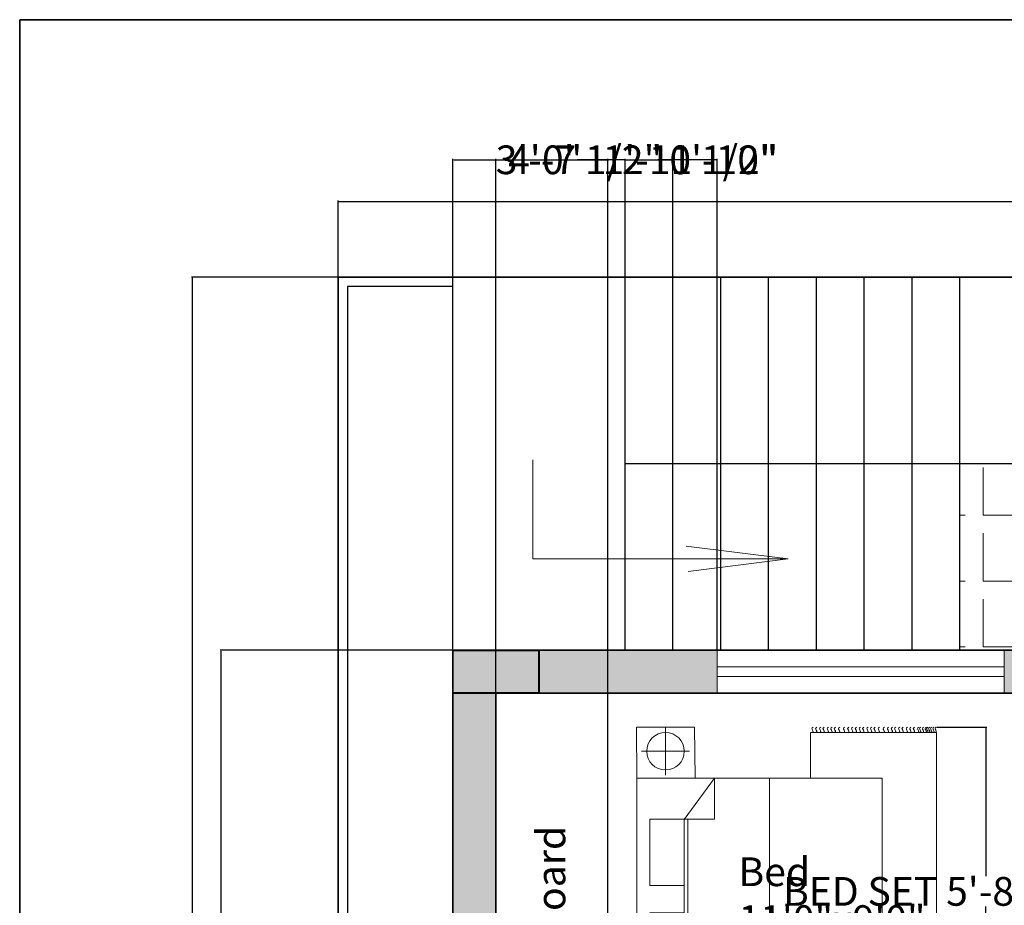
# Model space of a CAD drawing. Units: inches. Extents: x 56944 to 57417, y 173916 to 174454.
# Tile 7 of 8: x 56944 to 57149, y 174268 to 174454. Entities that reach past the tile are written whole.
import ezdxf

# ---------------------------------------------------------------- set-up
doc = ezdxf.new("R2010")
doc.units = ezdxf.units.IN
doc.header["$MEASUREMENT"] = 0
for name, color, linetype, lineweight in [('A-ANNO-DIMS', 2, 'Continuous', 18), ('A-ANNO-SYMB', 7, 'Continuous', 18), ('A-ANNO-TEXT', 7, 'Continuous', 18), ('A-ANNO-TTLB', 7, 'Continuous', 35), ('A-AREA-IDEN', 7, 'Continuous', 20), ('A-COLS', 7, 'Continuous', 40), ('A-COLS-PATT', 250, 'Continuous', 9), ('A-FLOR-CASE', 8, 'Continuous', 25), ('A-FLOR-STRS', 7, 'Continuous', 25), ('A-FURN', 8, 'Continuous', 18), ('A-GLAZ', 4, 'Continuous', 18), ('A-SITE-PATT', 8, 'Continuous', 9), ('A-SITE-WALL', 7, 'Continuous', 25), ('A-WALL', 7, 'Continuous', 35), ('A-WALL-PATT', 241, 'Continuous', 9), ('C-PROP', 7, 'Continuous', 35)]:
    doc.layers.add(name, color=color, linetype=linetype, lineweight=lineweight)
doc.styles.get("Standard").update_dxf_attribs({"font": 'arial.ttf'})
doc.dimstyles.get("Standard").update_dxf_attribs({"dimtxt": 6, "dimasz": 0.18, "dimexe": 0.18, "dimexo": 0.0625, "dimgap": 0.09, "dimtad": 0, "dimtih": 1, "dimtoh": 1, "dimdec": 1, "dimzin": 0, "dimdsep": 46, "dimlunit": 3, "dimtxsty": 'Standard', "dimcen": 0.09, "dimadec": 0, "dimazin": 0, "dimtfac": 1, "dimtdec": 1, "dimtofl": 0, "dimtmove": 0, "dimatfit": 3, "dimfxl": 1, "dimtolj": 1, "dimtzin": 0, "dimarcsym": 0})

# ---------------------------------------------------------------- blocks, each defined once
blk = doc.blocks.new('*D3')
at = {"layer": 'A-ANNO-DIMS', "color": 0, "lineweight": -2, "transparency": 16777216}
for p, q in [((57010.13, 174399.89), (57010.13, 174415.81)), ((57368.63, 174399.89), (57368.63, 174415.81)), ((57010.31, 174415.63), (57184.2, 174415.63)), ((57368.45, 174415.63), (57194.56, 174415.63))]:
    blk.add_line(p, q, dxfattribs=at)
at = {"layer": 'A-ANNO-DIMS', "color": 0, "transparency": 16777216}
for points in [[(57010.31, 174415.66), (57010.31, 174415.6), (57010.13, 174415.63)], [(57368.45, 174415.66), (57368.45, 174415.6), (57368.63, 174415.63)]]:
    blk.add_solid(points, dxfattribs=at)
at = {"layer": 'Defpoints', "color": 0, "transparency": 16777216}
for p in [(57368.63, 174415.63), (57010.13, 174399.82), (57368.63, 174399.82)]:
    blk.add_point(p, dxfattribs=at)
at = {"layer": 'A-ANNO-DIMS', "color": 0, "transparency": 16777216, "insert": (57189.38, 174415.63), "char_height": 6, "attachment_point": 5}
blk.add_mtext("\\A1;30'", dxfattribs=at)
blk = doc.blocks.new('*D4')
at = {"layer": 'A-ANNO-DIMS', "color": 0, "lineweight": -2, "transparency": 16777216}
for p, q in [((57010.07, 174399.82), (56979.48, 174399.82)), ((56979.66, 174399.64), (56979.66, 174183.23)), ((56979.66, 173960.5), (56979.66, 174176.92)), ((57010.07, 173960.32), (56979.48, 173960.32))]:
    blk.add_line(p, q, dxfattribs=at)
at = {"layer": 'A-ANNO-DIMS', "color": 0, "transparency": 16777216}
for points in [[(56979.63, 174399.64), (56979.69, 174399.64), (56979.66, 174399.82)], [(56979.63, 173960.5), (56979.69, 173960.5), (56979.66, 173960.32)]]:
    blk.add_solid(points, dxfattribs=at)
at = {"layer": 'Defpoints', "color": 0, "transparency": 16777216}
for p in [(57010.13, 174399.82), (56979.66, 173960.32), (57010.13, 173960.32)]:
    blk.add_point(p, dxfattribs=at)
at = {"layer": 'A-ANNO-DIMS', "color": 0, "transparency": 16777216, "insert": (56979.66, 174180.07), "char_height": 6, "width": 27.5975, "attachment_point": 5}
blk.add_mtext("\\A1;40'", dxfattribs=at)
blk = doc.blocks.new('BED-DOUBLE-WITH-NIGHTSTANDS')
for p, q in [((6.09, 68.68), (6.09, 58.62)), ((36.42, 67.59), (62.78, 67.59)), ((36.42, 58.05), (36.42, 67.59)), ((62.78, 67.59), (62.78, 4.35)), ((1.07, 63.65), (11.12, 63.65)), ((9.97, 49.39), (16.32, 58)), ((16.32, 49.44), (16.32, 58)), ((27.82, 58.05), (27.82, 10.63)), ((9.97, 49.44), (16.32, 49.44)), ((10.78, 49.44), (10.78, 10.63)), ((9.97, 49.39), (9.97, 10.63)), ((6.2, 10.63), (6.2, 0.57)), ((36.42, 4.35), (36.42, 10.65)), ((1.17, 5.6), (11.22, 5.6)), ((62.78, 4.35), (36.42, 4.35))]:
    blk.add_line(p, q)
for points in [[(12.29, 58.05), (12.19, 68.68), (0, 68.68), (0.1, 58.05)], [(0.1, 58.05), (51.42, 58.05), (51.42, 10.63), (0.1, 10.63)], [(2.8, 49.44), (9.97, 49.44), (9.97, 35.55), (2.8, 35.55)], [(2.8, 29.88), (9.97, 29.88), (9.97, 15.98), (2.8, 15.98)], [(12.39, 0), (12.29, 10.63), (0.1, 10.63), (0.21, 0)]]:
    blk.add_lwpolyline(points, close=True)
for centre in [(6.09, 63.65), (6.2, 5.6)]:
    blk.add_circle(centre, 3.92)
for points, knots in [([(36.95, 68.71), (36.83, 68.61), (36.59, 68.42), (36.83, 68.08), (37, 67.8), (36.89, 67.65), (36.85, 67.58)], [0, 0, 0, 0, 0.400747, 0.791423, 1.067667, 1.29709, 1.29709, 1.29709, 1.29709]), ([(37.73, 68.71), (37.61, 68.61), (37.37, 68.42), (37.61, 68.08), (37.78, 67.8), (37.67, 67.65), (37.62, 67.58)], [0, 0, 0, 0, 0.400747, 0.791423, 1.067667, 1.29709, 1.29709, 1.29709, 1.29709]), ([(38.54, 68.71), (38.42, 68.61), (38.18, 68.42), (38.42, 68.08), (38.59, 67.8), (38.49, 67.65), (38.44, 67.58)], [0, 0, 0, 0, 0.400747, 0.791423, 1.067667, 1.29709, 1.29709, 1.29709, 1.29709]), ([(39.27, 68.71), (39.15, 68.61), (38.91, 68.42), (39.15, 68.08), (39.32, 67.8), (39.22, 67.65), (39.17, 67.58)], [0, 0, 0, 0, 0.400747, 0.791423, 1.067667, 1.29709, 1.29709, 1.29709, 1.29709]), ([(40.15, 68.71), (40.03, 68.61), (39.79, 68.42), (40.03, 68.08), (40.2, 67.8), (40.1, 67.65), (40.05, 67.58)], [0, 0, 0, 0, 0.400747, 0.791423, 1.067667, 1.29709, 1.29709, 1.29709, 1.29709]), ([(40.91, 68.71), (40.78, 68.61), (40.54, 68.42), (40.78, 68.08), (40.96, 67.8), (40.85, 67.65), (40.8, 67.58)], [0, 0, 0, 0, 0.400747, 0.791423, 1.067667, 1.29709, 1.29709, 1.29709, 1.29709]), ([(41.63, 68.71), (41.51, 68.61), (41.27, 68.42), (41.51, 68.08), (41.68, 67.8), (41.58, 67.65), (41.53, 67.58)], [0, 0, 0, 0, 0.400747, 0.791423, 1.067667, 1.29709, 1.29709, 1.29709, 1.29709]), ([(42.52, 68.71), (42.39, 68.61), (42.15, 68.42), (42.39, 68.08), (42.57, 67.8), (42.46, 67.65), (42.41, 67.58)], [0, 0, 0, 0, 0.400747, 0.791423, 1.067667, 1.29709, 1.29709, 1.29709, 1.29709]), ([(43.55, 68.71), (43.43, 68.61), (43.19, 68.42), (43.43, 68.08), (43.6, 67.8), (43.5, 67.65), (43.45, 67.58)], [0, 0, 0, 0, 0.400747, 0.791423, 1.067667, 1.29709, 1.29709, 1.29709, 1.29709]), ([(44.43, 68.71), (44.31, 68.61), (44.07, 68.42), (44.31, 68.08), (44.49, 67.8), (44.38, 67.65), (44.33, 67.58)], [0, 0, 0, 0, 0.400747, 0.791423, 1.067667, 1.29709, 1.29709, 1.29709, 1.29709]), ([(45.25, 68.71), (45.13, 68.61), (44.89, 68.42), (45.13, 68.08), (45.3, 67.8), (45.2, 67.65), (45.15, 67.58)], [0, 0, 0, 0, 0.400747, 0.791423, 1.067667, 1.29709, 1.29709, 1.29709, 1.29709]), ([(46.03, 68.71), (45.91, 68.61), (45.67, 68.42), (45.91, 68.08), (46.08, 67.8), (45.97, 67.65), (45.92, 67.58)], [0, 0, 0, 0, 0.400747, 0.791423, 1.067667, 1.29709, 1.29709, 1.29709, 1.29709]), ([(46.84, 68.71), (46.72, 68.61), (46.48, 68.42), (46.72, 68.08), (46.9, 67.8), (46.79, 67.65), (46.74, 67.58)], [0, 0, 0, 0, 0.400747, 0.791423, 1.067667, 1.29709, 1.29709, 1.29709, 1.29709]), ([(47.57, 68.71), (47.45, 68.61), (47.21, 68.42), (47.45, 68.08), (47.62, 67.8), (47.52, 67.65), (47.47, 67.58)], [0, 0, 0, 0, 0.400747, 0.791423, 1.067667, 1.29709, 1.29709, 1.29709, 1.29709]), ([(48.45, 68.71), (48.33, 68.61), (48.09, 68.42), (48.33, 68.08), (48.51, 67.8), (48.4, 67.65), (48.35, 67.58)], [0, 0, 0, 0, 0.400747, 0.791423, 1.067667, 1.29709, 1.29709, 1.29709, 1.29709]), ([(49.21, 68.71), (49.08, 68.61), (48.85, 68.42), (49.08, 68.08), (49.26, 67.8), (49.15, 67.65), (49.1, 67.58)], [0, 0, 0, 0, 0.400747, 0.791423, 1.067667, 1.29709, 1.29709, 1.29709, 1.29709]), ([(49.93, 68.71), (49.81, 68.61), (49.57, 68.42), (49.81, 68.08), (49.99, 67.8), (49.88, 67.65), (49.83, 67.58)], [0, 0, 0, 0, 0.400747, 0.791423, 1.067667, 1.29709, 1.29709, 1.29709, 1.29709]), ([(50.82, 68.71), (50.69, 68.61), (50.46, 68.42), (50.69, 68.08), (50.87, 67.8), (50.76, 67.65), (50.71, 67.58)], [0, 0, 0, 0, 0.400747, 0.791423, 1.067667, 1.29709, 1.29709, 1.29709, 1.29709]), ([(51.85, 68.71), (51.73, 68.61), (51.49, 68.42), (51.73, 68.08), (51.9, 67.8), (51.8, 67.65), (51.75, 67.58)], [0, 0, 0, 0, 0.400747, 0.791423, 1.067667, 1.29709, 1.29709, 1.29709, 1.29709]), ([(52.73, 68.71), (52.61, 68.61), (52.37, 68.42), (52.61, 68.08), (52.79, 67.8), (52.68, 67.65), (52.63, 67.58)], [0, 0, 0, 0, 0.400747, 0.791423, 1.067667, 1.29709, 1.29709, 1.29709, 1.29709]), ([(53.55, 68.71), (53.43, 68.61), (53.19, 68.42), (53.43, 68.08), (53.6, 67.8), (53.5, 67.65), (53.45, 67.58)], [0, 0, 0, 0, 0.400747, 0.791423, 1.067667, 1.29709, 1.29709, 1.29709, 1.29709]), ([(54.24, 68.71), (54.12, 68.61), (53.88, 68.42), (54.12, 68.08), (54.29, 67.8), (54.19, 67.65), (54.14, 67.58)], [0, 0, 0, 0, 0.400747, 0.791423, 1.067667, 1.29709, 1.29709, 1.29709, 1.29709]), ([(55.06, 68.71), (54.94, 68.61), (54.7, 68.42), (54.94, 68.08), (55.11, 67.8), (55, 67.65), (54.95, 67.58)], [0, 0, 0, 0, 0.400747, 0.791423, 1.067667, 1.29709, 1.29709, 1.29709, 1.29709]), ([(55.78, 68.71), (55.66, 68.61), (55.42, 68.42), (55.66, 68.08), (55.84, 67.8), (55.73, 67.65), (55.68, 67.58)], [0, 0, 0, 0, 0.400747, 0.791423, 1.067667, 1.29709, 1.29709, 1.29709, 1.29709]), ([(56.67, 68.71), (56.55, 68.61), (56.31, 68.42), (56.55, 68.08), (56.72, 67.8), (56.61, 67.65), (56.56, 67.58)], [0, 0, 0, 0, 0.400747, 0.791423, 1.067667, 1.29709, 1.29709, 1.29709, 1.29709]), ([(57.42, 68.71), (57.3, 68.61), (57.06, 68.42), (57.3, 68.08), (57.47, 67.8), (57.36, 67.65), (57.32, 67.58)], [0, 0, 0, 0, 0.400747, 0.791423, 1.067667, 1.29709, 1.29709, 1.29709, 1.29709]), ([(58.15, 68.71), (58.03, 68.61), (57.79, 68.42), (58.03, 68.08), (58.2, 67.8), (58.1, 67.66), (58.05, 67.59)], [0, 0, 0, 0, 0.400747, 0.791423, 1.067667, 1.283686, 1.283686, 1.283686, 1.283686]), ([(59.03, 68.71), (58.91, 68.61), (58.67, 68.42), (58.91, 68.08), (59.08, 67.8), (58.98, 67.66), (58.93, 67.59)], [0, 0, 0, 0, 0.400747, 0.791423, 1.067667, 1.283686, 1.283686, 1.283686, 1.283686]), ([(59.46, 68.71), (59.34, 68.61), (59.09, 68.42), (59.34, 68.08), (59.51, 67.8), (59.41, 67.66), (59.36, 67.59)], [0, 0, 0, 0, 0.402903, 0.794912, 1.071156, 1.287177, 1.287177, 1.287177, 1.287177]), ([(60.05, 68.71), (59.93, 68.61), (59.69, 68.42), (59.93, 68.08), (60.1, 67.8), (60, 67.66), (59.96, 67.59)], [0, 0, 0, 0, 0.400747, 0.791423, 1.067667, 1.283686, 1.283686, 1.283686, 1.283686]), ([(60.63, 68.71), (60.51, 68.61), (60.27, 68.42), (60.51, 68.08), (60.68, 67.8), (60.58, 67.66), (60.53, 67.59)], [0, 0, 0, 0, 0.400747, 0.791423, 1.067667, 1.283686, 1.283686, 1.283686, 1.283686]), ([(60.94, 68.71), (60.82, 68.61), (60.58, 68.42), (60.81, 68.08), (60.99, 67.8), (60.89, 67.66), (60.84, 67.59)], [0, 0, 0, 0, 0.400747, 0.791423, 1.067667, 1.283686, 1.283686, 1.283686, 1.283686]), ([(61.35, 68.71), (61.23, 68.61), (60.99, 68.42), (61.23, 68.08), (61.41, 67.8), (61.3, 67.65), (61.25, 67.58)], [0, 0, 0, 0, 0.400747, 0.791423, 1.067667, 1.29709, 1.29709, 1.29709, 1.29709]), ([(61.75, 68.71), (61.63, 68.61), (61.39, 68.42), (61.63, 68.08), (61.8, 67.8), (61.7, 67.65), (61.65, 67.58)], [0, 0, 0, 0, 0.400747, 0.791423, 1.067667, 1.29709, 1.29709, 1.29709, 1.29709]), ([(62.24, 68.71), (62.12, 68.61), (61.88, 68.42), (62.12, 68.08), (62.29, 67.8), (62.18, 67.65), (62.13, 67.58)], [0, 0, 0, 0, 0.400747, 0.791423, 1.067667, 1.29709, 1.29709, 1.29709, 1.29709]), ([(62.71, 68.71), (62.59, 68.61), (62.35, 68.42), (62.59, 68.08), (62.76, 67.8), (62.66, 67.65), (62.61, 67.58)], [0, 0, 0, 0, 0.400747, 0.791423, 1.067667, 1.29709, 1.29709, 1.29709, 1.29709]), ([(36.95, 3.23), (36.83, 3.32), (36.59, 3.52), (36.83, 3.86), (37, 4.14), (36.89, 4.29), (36.85, 4.35)], [0, 0, 0, 0, 0.400747, 0.791423, 1.067667, 1.29709, 1.29709, 1.29709, 1.29709]), ([(37.73, 3.23), (37.61, 3.32), (37.37, 3.52), (37.61, 3.86), (37.78, 4.14), (37.67, 4.29), (37.62, 4.35)], [0, 0, 0, 0, 0.400747, 0.791423, 1.067667, 1.29709, 1.29709, 1.29709, 1.29709]), ([(38.54, 3.23), (38.42, 3.32), (38.18, 3.52), (38.42, 3.86), (38.59, 4.14), (38.49, 4.29), (38.44, 4.35)], [0, 0, 0, 0, 0.400747, 0.791423, 1.067667, 1.29709, 1.29709, 1.29709, 1.29709]), ([(39.27, 3.23), (39.15, 3.32), (38.91, 3.52), (39.15, 3.86), (39.32, 4.14), (39.22, 4.29), (39.17, 4.35)], [0, 0, 0, 0, 0.400747, 0.791423, 1.067667, 1.29709, 1.29709, 1.29709, 1.29709]), ([(40.15, 3.23), (40.03, 3.32), (39.79, 3.52), (40.03, 3.86), (40.2, 4.14), (40.1, 4.29), (40.05, 4.35)], [0, 0, 0, 0, 0.400747, 0.791423, 1.067667, 1.29709, 1.29709, 1.29709, 1.29709]), ([(40.91, 3.23), (40.78, 3.32), (40.54, 3.52), (40.78, 3.86), (40.96, 4.14), (40.85, 4.29), (40.8, 4.35)], [0, 0, 0, 0, 0.400747, 0.791423, 1.067667, 1.29709, 1.29709, 1.29709, 1.29709]), ([(41.63, 3.23), (41.51, 3.32), (41.27, 3.52), (41.51, 3.86), (41.68, 4.14), (41.58, 4.29), (41.53, 4.35)], [0, 0, 0, 0, 0.400747, 0.791423, 1.067667, 1.29709, 1.29709, 1.29709, 1.29709]), ([(42.52, 3.23), (42.39, 3.32), (42.15, 3.52), (42.39, 3.86), (42.57, 4.14), (42.46, 4.29), (42.41, 4.35)], [0, 0, 0, 0, 0.400747, 0.791423, 1.067667, 1.29709, 1.29709, 1.29709, 1.29709]), ([(43.55, 3.23), (43.43, 3.32), (43.19, 3.52), (43.43, 3.86), (43.6, 4.14), (43.5, 4.29), (43.45, 4.35)], [0, 0, 0, 0, 0.400747, 0.791423, 1.067667, 1.29709, 1.29709, 1.29709, 1.29709]), ([(44.43, 3.23), (44.31, 3.32), (44.07, 3.52), (44.31, 3.86), (44.49, 4.14), (44.38, 4.29), (44.33, 4.35)], [0, 0, 0, 0, 0.400747, 0.791423, 1.067667, 1.29709, 1.29709, 1.29709, 1.29709]), ([(45.25, 3.23), (45.13, 3.32), (44.89, 3.52), (45.13, 3.86), (45.3, 4.14), (45.2, 4.29), (45.15, 4.35)], [0, 0, 0, 0, 0.400747, 0.791423, 1.067667, 1.29709, 1.29709, 1.29709, 1.29709]), ([(46.03, 3.23), (45.91, 3.32), (45.67, 3.52), (45.91, 3.86), (46.08, 4.14), (45.97, 4.29), (45.92, 4.35)], [0, 0, 0, 0, 0.400747, 0.791423, 1.067667, 1.29709, 1.29709, 1.29709, 1.29709]), ([(46.84, 3.23), (46.72, 3.32), (46.48, 3.52), (46.72, 3.86), (46.9, 4.14), (46.79, 4.29), (46.74, 4.35)], [0, 0, 0, 0, 0.400747, 0.791423, 1.067667, 1.29709, 1.29709, 1.29709, 1.29709]), ([(47.57, 3.23), (47.45, 3.32), (47.21, 3.52), (47.45, 3.86), (47.62, 4.14), (47.52, 4.29), (47.47, 4.35)], [0, 0, 0, 0, 0.400747, 0.791423, 1.067667, 1.29709, 1.29709, 1.29709, 1.29709]), ([(48.45, 3.23), (48.33, 3.32), (48.09, 3.52), (48.33, 3.86), (48.51, 4.14), (48.4, 4.29), (48.35, 4.35)], [0, 0, 0, 0, 0.400747, 0.791423, 1.067667, 1.29709, 1.29709, 1.29709, 1.29709]), ([(49.21, 3.23), (49.08, 3.32), (48.85, 3.52), (49.08, 3.86), (49.26, 4.14), (49.15, 4.29), (49.1, 4.35)], [0, 0, 0, 0, 0.400747, 0.791423, 1.067667, 1.29709, 1.29709, 1.29709, 1.29709]), ([(49.93, 3.23), (49.81, 3.32), (49.57, 3.52), (49.81, 3.86), (49.99, 4.14), (49.88, 4.29), (49.83, 4.35)], [0, 0, 0, 0, 0.400747, 0.791423, 1.067667, 1.29709, 1.29709, 1.29709, 1.29709]), ([(50.82, 3.23), (50.69, 3.32), (50.46, 3.52), (50.69, 3.86), (50.87, 4.14), (50.76, 4.29), (50.71, 4.35)], [0, 0, 0, 0, 0.400747, 0.791423, 1.067667, 1.29709, 1.29709, 1.29709, 1.29709]), ([(51.85, 3.23), (51.73, 3.32), (51.49, 3.52), (51.73, 3.86), (51.9, 4.14), (51.8, 4.29), (51.75, 4.35)], [0, 0, 0, 0, 0.400747, 0.791423, 1.067667, 1.29709, 1.29709, 1.29709, 1.29709]), ([(52.73, 3.23), (52.61, 3.32), (52.37, 3.52), (52.61, 3.86), (52.79, 4.14), (52.68, 4.29), (52.63, 4.35)], [0, 0, 0, 0, 0.400747, 0.791423, 1.067667, 1.29709, 1.29709, 1.29709, 1.29709]), ([(53.55, 3.23), (53.43, 3.32), (53.19, 3.52), (53.43, 3.86), (53.6, 4.14), (53.5, 4.29), (53.45, 4.35)], [0, 0, 0, 0, 0.400747, 0.791423, 1.067667, 1.29709, 1.29709, 1.29709, 1.29709]), ([(54.24, 3.23), (54.12, 3.32), (53.88, 3.52), (54.12, 3.86), (54.29, 4.14), (54.19, 4.29), (54.14, 4.35)], [0, 0, 0, 0, 0.400747, 0.791423, 1.067667, 1.29709, 1.29709, 1.29709, 1.29709]), ([(55.06, 3.23), (54.94, 3.32), (54.7, 3.52), (54.94, 3.86), (55.11, 4.14), (55, 4.29), (54.95, 4.35)], [0, 0, 0, 0, 0.400747, 0.791423, 1.067667, 1.29709, 1.29709, 1.29709, 1.29709]), ([(55.78, 3.23), (55.66, 3.32), (55.42, 3.52), (55.66, 3.86), (55.84, 4.14), (55.73, 4.29), (55.68, 4.35)], [0, 0, 0, 0, 0.400747, 0.791423, 1.067667, 1.29709, 1.29709, 1.29709, 1.29709]), ([(56.67, 3.23), (56.55, 3.32), (56.31, 3.52), (56.55, 3.86), (56.72, 4.14), (56.61, 4.29), (56.56, 4.35)], [0, 0, 0, 0, 0.400747, 0.791423, 1.067667, 1.29709, 1.29709, 1.29709, 1.29709]), ([(57.42, 3.23), (57.3, 3.32), (57.06, 3.52), (57.3, 3.86), (57.47, 4.14), (57.36, 4.29), (57.32, 4.35)], [0, 0, 0, 0, 0.400747, 0.791423, 1.067667, 1.29709, 1.29709, 1.29709, 1.29709]), ([(58.15, 3.23), (58.03, 3.32), (57.79, 3.52), (58.03, 3.86), (58.2, 4.14), (58.09, 4.29), (58.04, 4.35)], [0, 0, 0, 0, 0.400747, 0.791423, 1.067667, 1.29709, 1.29709, 1.29709, 1.29709]), ([(59.03, 3.23), (58.91, 3.32), (58.67, 3.52), (58.91, 3.86), (59.08, 4.14), (58.97, 4.29), (58.93, 4.35)], [0, 0, 0, 0, 0.400747, 0.791423, 1.067667, 1.29709, 1.29709, 1.29709, 1.29709]), ([(59.46, 3.23), (59.33, 3.32), (59.08, 3.51), (59.34, 3.86), (59.51, 4.14), (59.4, 4.29), (59.36, 4.35)], [0, 0, 0, 0, 0.407265, 0.802015, 1.07826, 1.307683, 1.307683, 1.307683, 1.307683]), ([(60.03, 3.23), (59.9, 3.32), (59.67, 3.52), (59.9, 3.86), (60.08, 4.14), (59.97, 4.29), (59.92, 4.35)], [0, 0, 0, 0, 0.400747, 0.791423, 1.067667, 1.29709, 1.29709, 1.29709, 1.29709]), ([(60.6, 3.23), (60.48, 3.32), (60.24, 3.52), (60.48, 3.86), (60.65, 4.14), (60.54, 4.29), (60.5, 4.35)], [0, 0, 0, 0, 0.400747, 0.791423, 1.067667, 1.29709, 1.29709, 1.29709, 1.29709]), ([(60.91, 3.23), (60.79, 3.32), (60.55, 3.52), (60.79, 3.86), (60.96, 4.14), (60.85, 4.29), (60.81, 4.35)], [0, 0, 0, 0, 0.400747, 0.791423, 1.067667, 1.29709, 1.29709, 1.29709, 1.29709]), ([(61.33, 3.23), (61.21, 3.32), (60.97, 3.52), (61.21, 3.86), (61.38, 4.14), (61.27, 4.29), (61.22, 4.35)], [0, 0, 0, 0, 0.400747, 0.791423, 1.067667, 1.29709, 1.29709, 1.29709, 1.29709]), ([(61.72, 3.23), (61.6, 3.32), (61.36, 3.52), (61.6, 3.86), (61.78, 4.14), (61.67, 4.29), (61.62, 4.35)], [0, 0, 0, 0, 0.400747, 0.791423, 1.067667, 1.29709, 1.29709, 1.29709, 1.29709]), ([(62.21, 3.23), (62.09, 3.32), (61.85, 3.52), (62.09, 3.86), (62.26, 4.14), (62.15, 4.29), (62.11, 4.35)], [0, 0, 0, 0, 0.400747, 0.791423, 1.067667, 1.29709, 1.29709, 1.29709, 1.29709]), ([(62.71, 3.23), (62.59, 3.32), (62.35, 3.52), (62.59, 3.86), (62.76, 4.14), (62.66, 4.29), (62.61, 4.35)], [0, 0, 0, 0, 0.400747, 0.791423, 1.067667, 1.29709, 1.29709, 1.29709, 1.29709])]:
    blk.add_open_spline(points, degree=3, knots=knots)
blk = doc.blocks.new('GLAZ-LITE-60IN')
for p, q in [((0, 2), (60, 2)), ((60, 0), (0, 0))]:
    blk.add_line(p, q)
blk = doc.blocks.new('*D16')
at = {"layer": 'A-ANNO-DIMS', "color": 0, "lineweight": -2, "transparency": 16777216}
for p, q in [((57135.34, 174305.75), (57145.76, 174305.75)), ((57145.58, 174305.57), (57145.58, 174274.59)), ((57145.58, 174237.22), (57145.58, 174268.2)), ((57135.34, 174237.04), (57145.76, 174237.04))]:
    blk.add_line(p, q, dxfattribs=at)
at = {"layer": 'A-ANNO-DIMS', "color": 0, "transparency": 16777216}
for points in [[(57145.55, 174305.57), (57145.61, 174305.57), (57145.58, 174305.75)], [(57145.55, 174237.22), (57145.61, 174237.22), (57145.58, 174237.04)]]:
    blk.add_solid(points, dxfattribs=at)
at = {"layer": 'Defpoints', "color": 0, "transparency": 16777216}
for p in [(57135.28, 174305.75), (57145.58, 174305.75), (57135.28, 174237.04)]:
    blk.add_point(p, dxfattribs=at)
at = {"layer": 'A-ANNO-DIMS', "color": 0, "transparency": 16777216, "insert": (57145.58, 174271.39), "char_height": 6, "attachment_point": 5}
blk.add_mtext('\\A1;BED SET 5\'-8 1/2" TYP.', dxfattribs=at)
blk = doc.blocks.new('*D37')
at = {"layer": 'A-ANNO-DIMS', "color": 0, "lineweight": -2, "transparency": 16777216}
for p, q in [((57034.07, 174321.82), (56985.45, 174321.82)), ((56985.63, 174321.64), (56985.63, 174144.27)), ((56985.63, 173960.5), (56985.63, 174137.88)), ((57034.07, 173960.32), (56985.45, 173960.32))]:
    blk.add_line(p, q, dxfattribs=at)
at = {"layer": 'A-ANNO-DIMS', "color": 0, "transparency": 16777216}
for points in [[(56985.6, 174321.64), (56985.66, 174321.64), (56985.63, 174321.82)], [(56985.6, 173960.5), (56985.66, 173960.5), (56985.63, 173960.32)]]:
    blk.add_solid(points, dxfattribs=at)
at = {"layer": 'Defpoints', "color": 0, "transparency": 16777216}
for p in [(56985.63, 174321.82), (57034.13, 174321.82), (57034.13, 173960.32)]:
    blk.add_point(p, dxfattribs=at)
at = {"layer": 'A-ANNO-DIMS', "color": 0, "transparency": 16777216, "insert": (56985.63, 174141.07), "char_height": 6, "attachment_point": 5}
blk.add_mtext('\\A1;30\'-1 1/2"', dxfattribs=at)
blk = doc.blocks.new('*D38')
at = {"layer": 'A-ANNO-DIMS', "color": 0, "lineweight": -2, "transparency": 16777216}
for p, q in [((57070.13, 174399.89), (57070.13, 174424.5)), ((57070.31, 174424.32), (57079.95, 174424.32)), ((57080.13, 174399.89), (57080.13, 174424.5)), ((57080.13, 174424.32), (57080.31, 174424.32))]:
    blk.add_line(p, q, dxfattribs=at)
at = {"layer": 'A-ANNO-DIMS', "color": 0, "transparency": 16777216}
for points in [[(57070.31, 174424.35), (57070.31, 174424.29), (57070.13, 174424.32)], [(57079.95, 174424.35), (57079.95, 174424.29), (57080.13, 174424.32)]]:
    blk.add_solid(points, dxfattribs=at)
at = {"layer": 'Defpoints', "color": 0, "transparency": 16777216}
for p in [(57080.13, 174424.32), (57070.13, 174399.82), (57080.13, 174399.82)]:
    blk.add_point(p, dxfattribs=at)
at = {"layer": 'A-ANNO-DIMS', "color": 0, "transparency": 16777216, "insert": (57090.71, 174424.32), "char_height": 6, "attachment_point": 5}
blk.add_mtext('\\A1;0\'-10"', dxfattribs=at)
blk = doc.blocks.new('*D40')
at = {"layer": 'A-ANNO-DIMS', "color": 0, "lineweight": -2, "transparency": 16777216}
for p, q in [((57034.13, 174399.89), (57034.13, 174424.5)), ((57034.31, 174424.32), (57044.07, 174424.32)), ((57069.95, 174424.32), (57060.2, 174424.32)), ((57070.13, 174399.89), (57070.13, 174424.5))]:
    blk.add_line(p, q, dxfattribs=at)
at = {"layer": 'A-ANNO-DIMS', "color": 0, "transparency": 16777216}
for points in [[(57034.31, 174424.35), (57034.31, 174424.29), (57034.13, 174424.32)], [(57069.95, 174424.35), (57069.95, 174424.29), (57070.13, 174424.32)]]:
    blk.add_solid(points, dxfattribs=at)
at = {"layer": 'Defpoints', "color": 0, "transparency": 16777216}
for p in [(57070.13, 174424.32), (57034.13, 174399.82), (57070.13, 174399.82)]:
    blk.add_point(p, dxfattribs=at)
at = {"layer": 'A-ANNO-DIMS', "color": 0, "transparency": 16777216, "insert": (57052.13, 174424.32), "char_height": 6, "attachment_point": 5}
blk.add_mtext('\\A1;3\'-0"', dxfattribs=at)
blk = doc.blocks.new('*D42')
at = {"layer": 'A-ANNO-DIMS', "color": 0, "lineweight": -2, "transparency": 16777216}
for p, q in [((57043.13, 174312.89), (57043.13, 174424.5)), ((57043.31, 174424.32), (57066.33, 174424.32)), ((57066.51, 174312.89), (57066.51, 174424.5)), ((57066.51, 174424.32), (57066.69, 174424.32))]:
    blk.add_line(p, q, dxfattribs=at)
at = {"layer": 'A-ANNO-DIMS', "color": 0, "transparency": 16777216}
for points in [[(57043.31, 174424.35), (57043.31, 174424.29), (57043.13, 174424.32)], [(57066.33, 174424.35), (57066.33, 174424.29), (57066.51, 174424.32)]]:
    blk.add_solid(points, dxfattribs=at)
at = {"layer": 'Defpoints', "color": 0, "transparency": 16777216}
for p in [(57066.51, 174424.32), (57043.13, 174312.82), (57066.51, 174312.82)]:
    blk.add_point(p, dxfattribs=at)
at = {"layer": 'A-ANNO-DIMS', "color": 0, "transparency": 16777216, "insert": (57083.8, 174424.32), "char_height": 6, "attachment_point": 5}
blk.add_mtext('\\A1;1\'-11 1/2"', dxfattribs=at)
blk = doc.blocks.new('*D55')
at = {"layer": 'A-ANNO-DIMS', "color": 0, "lineweight": -2, "transparency": 16777216}
for p, q in [((57034.13, 174321.89), (57034.13, 174424.5)), ((57034.31, 174424.32), (57046.6, 174424.32)), ((57089.24, 174424.32), (57076.95, 174424.32)), ((57089.42, 174321.89), (57089.42, 174424.5))]:
    blk.add_line(p, q, dxfattribs=at)
at = {"layer": 'A-ANNO-DIMS', "color": 0, "transparency": 16777216}
for points in [[(57034.31, 174424.35), (57034.31, 174424.29), (57034.13, 174424.32)], [(57089.24, 174424.35), (57089.24, 174424.29), (57089.42, 174424.32)]]:
    blk.add_solid(points, dxfattribs=at)
at = {"layer": 'Defpoints', "color": 0, "transparency": 16777216}
for p in [(57089.42, 174424.32), (57034.13, 174321.82), (57089.42, 174321.82)]:
    blk.add_point(p, dxfattribs=at)
at = {"layer": 'A-ANNO-DIMS', "color": 0, "transparency": 16777216, "insert": (57061.78, 174424.32), "char_height": 6, "attachment_point": 5}
blk.add_mtext('\\A1;4\'-7 1/2"', dxfattribs=at)

msp = doc.modelspace()

# ---------------------------------------------------------------- hatches: boundary and pattern name
at = {"layer": 'A-COLS-PATT'}
h = msp.add_hatch(color=256, dxfattribs=at)
h.dxf.hatch_style = 1
h.paths.add_polyline_path([(57052.13, 174321.82), (57034.13, 174321.82), (57034.13, 174312.82), (57052.13, 174312.82)])
h.paths.add_polyline_path([(57186.38, 174321.82), (57168.38, 174321.82), (57168.38, 174312.82), (57175.13, 174312.82), (57186.38, 174312.82)])
h.paths.add_polyline_path([(57308.63, 174321.82), (57290.63, 174321.82), (57290.63, 174312.82), (57308.63, 174312.82)])
h.paths.add_polyline_path([(57179.63, 174204.82), (57170.63, 174204.82), (57170.63, 174186.82), (57179.63, 174186.82)])
h.paths.add_polyline_path([(57043.13, 174204.82), (57034.13, 174204.82), (57034.13, 174186.82), (57043.13, 174186.82)])
h.paths.add_polyline_path([(57308.63, 174206.32), (57299.63, 174206.32), (57299.63, 174188.32), (57308.63, 174188.32)])
h.paths.add_polyline_path([(57308.63, 174107.87), (57299.63, 174107.87), (57299.63, 174093.93), (57308.63, 174093.93)])
h.paths.add_polyline_path([(57308.63, 173978.32), (57299.63, 173978.32), (57299.63, 173960.32), (57308.63, 173960.32)])
h.paths.add_polyline_path([(57179.63, 173969.32), (57161.63, 173969.32), (57161.63, 173960.32), (57179.63, 173960.32)])
h.paths.add_polyline_path([(57043.13, 173978.32), (57034.13, 173978.32), (57034.13, 173960.32), (57043.13, 173960.32)])
h.paths.add_polyline_path([(57043.13, 174099.82), (57034.13, 174099.82), (57034.13, 174081.82), (57043.13, 174081.82)])
h.paths.add_polyline_path([(57179.63, 174099.82), (57170.63, 174099.82), (57170.63, 174081.82), (57179.63, 174081.82)])
at = {"layer": 'A-SITE-PATT'}
h = msp.add_hatch(dxfattribs=at)
h.set_pattern_fill('ANGLE', color=256, scale=50)
h.set_pattern_definition([(0, (0, 0), (0, 13.75), [10, -3.75]), (90, (0, 0), (-13.75, 8e-16), [10, -3.75])])
h.paths.add_polyline_path([(57365.63, 174396.82), (57200.13, 174396.82), (57200.13, 174379.18), (57215.46, 174379.18, -1.049383), (57218.84, 174379.34, -0.952941), (57215.46, 174379.18), (57200.13, 174379.18), (57200.13, 174360.82), (57140.13, 174360.82), (57140.13, 174321.82), (57149.42, 174321.82), (57243.2, 174321.82), (57282.32, 174321.82), (57283.32, 174321.82), (57308.63, 174321.82), (57308.63, 174305.82), (57308.63, 174259.72), (57308.63, 174258.72), (57308.63, 174252.72), (57308.63, 174216.72), (57308.63, 174099.82), (57308.63, 174093.93), (57308.63, 174081.93), (57308.63, 173969.32), (57365.63, 173969.32)])
h.paths.add_polyline_path([(57341.88, 174114.38), (57341.88, 174209.81), (57329.51, 174209.81), (57329.51, 174114.38)], flags=24)
h.paths.add_polyline_path([(57215.63, 174350.61), (57326.6, 174350.61), (57326.6, 174362.97), (57215.63, 174362.97)], flags=24)
at = {"layer": 'A-WALL-PATT'}
h = msp.add_hatch(color=256, dxfattribs=at)
h.dxf.hatch_style = 1
h.paths.add_polyline_path([(57089.42, 174321.82), (57052.13, 174321.82), (57052.13, 174312.82), (57089.42, 174312.82)])
h.paths.add_polyline_path([(57168.38, 174321.82), (57149.42, 174321.82), (57149.42, 174312.82), (57168.38, 174312.82)])
h.paths.add_polyline_path([(57199.66, 174321.82), (57186.38, 174321.82), (57186.38, 174312.82), (57199.66, 174312.82)])
h.paths.add_polyline_path([(57179.63, 174312.82), (57177.38, 174312.82), (57175.13, 174312.82), (57175.13, 174204.82), (57179.63, 174204.82)])
h.paths.add_polyline_path([(57043.13, 174312.82), (57034.13, 174312.82), (57034.13, 174204.82), (57043.13, 174204.82)])
h.paths.add_polyline_path([(57043.13, 174147.82), (57121.13, 174147.82), (57121.13, 174099.82), (57115.13, 174099.82), (57115.13, 174095.32), (57121.13, 174095.32), (57133.63, 174095.32), (57133.63, 174099.82), (57125.63, 174099.82), (57125.63, 174200.32), (57133.63, 174200.32), (57133.63, 174204.82), (57115.13, 174204.82), (57115.13, 174200.32), (57121.13, 174200.32), (57121.13, 174152.32), (57043.13, 174152.32), (57043.13, 174162.82), (57034.13, 174162.82), (57034.13, 174131.11), (57043.13, 174131.11)])
h.paths.add_polyline_path([(57043.13, 174081.82), (57034.13, 174081.82), (57034.13, 173978.32), (57043.13, 173978.32)])
h.paths.add_polyline_path([(57093.93, 173969.32), (57043.13, 173969.32), (57043.13, 173960.32), (57093.93, 173960.32)])
h.paths.add_polyline_path([(57161.63, 173969.32), (57153.93, 173969.32), (57153.93, 173960.32), (57161.63, 173960.32)])
h.paths.add_polyline_path([(57179.63, 174081.82), (57175.13, 174081.82), (57175.13, 173969.32), (57179.63, 173969.32)])
h.paths.add_polyline_path([(57299.63, 173969.32), (57179.63, 173969.32), (57179.63, 173960.32), (57299.63, 173960.32)])
h.paths.add_polyline_path([(57308.63, 174025.05), (57299.63, 174025.05), (57299.63, 173978.32), (57308.63, 173978.32)])
h.paths.add_polyline_path([(57308.63, 174081.93), (57299.63, 174081.93), (57299.63, 174075.82), (57227.63, 174075.82), (57227.63, 174081.82), (57223.13, 174081.82), (57223.13, 174075.82), (57223.13, 174071.32), (57299.63, 174071.32), (57299.63, 174061.05), (57308.63, 174061.05)])
h.paths.add_polyline_path([(57308.63, 174140.51), (57299.63, 174140.51), (57299.63, 174128.32), (57223.13, 174128.32), (57223.13, 174117.82), (57227.63, 174117.82), (57227.63, 174123.82), (57299.63, 174123.82), (57299.63, 174119.87), (57308.63, 174119.87)])
h.paths.add_polyline_path([(57308.63, 174216.72), (57299.63, 174216.72), (57299.63, 174206.32), (57308.63, 174206.32)])
h.paths.add_polyline_path([(57308.63, 174188.32), (57299.63, 174188.32), (57299.63, 174176.51), (57308.63, 174176.51)])
h.paths.add_polyline_path([(57308.63, 174258.72), (57299.63, 174258.72), (57299.63, 174252.72), (57308.63, 174252.72)])
h.paths.add_polyline_path([(57308.63, 174312.82), (57299.63, 174312.82), (57299.63, 174306.82), (57308.63, 174306.82)])
h.paths.add_polyline_path([(57290.63, 174321.82), (57283.32, 174321.82), (57283.32, 174312.82), (57290.63, 174312.82)])
h.paths.add_polyline_path([(57242.2, 174321.82), (57235.66, 174321.82), (57235.66, 174312.82), (57242.2, 174312.82)])
h.paths.add_polyline_path([(57083.13, 174204.82), (57043.13, 174204.82), (57043.13, 174200.32), (57083.13, 174200.32)], flags=17)
h.paths.add_polyline_path([(57083.13, 174099.82), (57043.13, 174099.82), (57043.13, 174095.32), (57083.13, 174095.32)], flags=0)

# ---------------------------------------------------------------- linework, layer by layer
at = {"layer": 'A-ANNO-SYMB'}
for p, q in [((57050.87, 174361.59), (57050.87, 174340.93)), ((57104.22, 174340.93), (57082.93, 174343.54)), ((57082.93, 174343.54), (57104.22, 174340.93)), ((57050.87, 174340.93), (57104.22, 174340.93)), ((57104.22, 174340.93), (57083.33, 174338.23))]:
    msp.add_line(p, q, dxfattribs=at)
at = {"layer": 'A-ANNO-TTLB'}
msp.add_lwpolyline([(56943.57, 174453.61), (57416.55, 174453.61), (57416.55, 173915.6), (56943.57, 173915.6)], close=True, dxfattribs=at)
at = {"layer": 'A-COLS'}
for p, q in [((57034.13, 174321.82), (57052.13, 174321.82)), ((57052.13, 174321.82), (57052.13, 174312.82)), ((57052.13, 174312.82), (57034.13, 174312.82))]:
    msp.add_line(p, q, dxfattribs=at)
at = {"layer": 'A-FLOR-CASE'}
msp.add_line((57066.51, 174204.82), (57066.51, 174312.82), dxfattribs=at)
at = {"layer": 'A-FLOR-STRS'}
for p, q in [((57034.13, 174321.82), (57034.13, 174399.82)), ((57070.13, 174321.82), (57070.13, 174399.82)), ((57080.13, 174321.82), (57080.13, 174399.82)), ((57090.13, 174321.82), (57090.13, 174399.82)), ((57100.13, 174321.82), (57100.13, 174399.82)), ((57110.13, 174321.82), (57110.13, 174399.82)), ((57120.13, 174321.82), (57120.13, 174399.82)), ((57130.13, 174321.82), (57130.13, 174399.82)), ((57140.13, 174321.82), (57140.13, 174399.82)), ((57070.13, 174360.82), (57200.13, 174360.82)), ((57034.13, 174321.82), (57070.13, 174321.82))]:
    msp.add_line(p, q, dxfattribs=at)
at = {"layer": 'A-GLAZ'}
for p, q in [((57089.42, 174312.82), (57089.42, 174321.82)), ((57089.42, 174321.82), (57149.42, 174321.82)), ((57149.42, 174321.82), (57149.42, 174312.82)), ((57149.42, 174312.82), (57089.42, 174312.82))]:
    msp.add_line(p, q, dxfattribs=at)
at = {"layer": 'A-SITE-WALL'}
for p, q in [((57034.13, 174397.82), (57012.13, 174397.82)), ((57012.13, 174397.82), (57012.13, 173960.32))]:
    msp.add_line(p, q, dxfattribs=at)
at = {"layer": 'A-WALL'}
for p, q in [((57034.13, 174321.82), (57243.2, 174321.82)), ((57034.13, 174321.82), (57034.13, 173960.32)), ((57034.13, 174312.82), (57242.2, 174312.82)), ((57043.13, 174312.82), (57043.13, 174152.32))]:
    msp.add_line(p, q, dxfattribs=at)
at = {"layer": 'C-PROP'}
for p, q in [((57034.13, 174399.82), (57010.13, 174399.82)), ((57010.13, 174399.82), (57010.13, 173960.32)), ((57034.13, 174399.82), (57308.63, 174399.82))]:
    msp.add_line(p, q, dxfattribs=at)

# ---------------------------------------------------------------- block references
at = {"layer": 'A-FURN'}
msp.add_blockref('BED-DOUBLE-WITH-NIGHTSTANDS', (57072.49, 174237.04), dxfattribs=at)
at = {"layer": 'A-GLAZ'}
msp.add_blockref('GLAZ-LITE-60IN', (57089.42, 174316.32), dxfattribs=at)

# ---------------------------------------------------------------- texts
at = {"layer": 'A-ANNO-TEXT', "insert": (57051.64, 174245.19), "char_height": 6, "attachment_point": 1, "rotation": 90}
msp.add_mtext_dynamic_manual_height_columns('cub-board', width=40.1458, gutter_width=1, heights=[0], dxfattribs=at)
at = {"layer": 'A-AREA-IDEN', "insert": (57093.84, 174278.49), "char_height": 6, "attachment_point": 1}
msp.add_mtext_dynamic_manual_height_columns('Bed \\P11\'0"x9\'0"', width=57.7195, gutter_width=1, heights=[0], dxfattribs=at)

# ---------------------------------------------------------------- dimensions: what is measured, and where the dimension line sits
at = {"layer": 'A-ANNO-DIMS'}
for base, p1, p2, picture, middle in [((57089.42, 174424.32), (57034.13, 174321.82), (57089.42, 174321.82), '*D55', (57061.78, 174424.32)), ((57066.51, 174424.32), (57043.13, 174312.82), (57066.51, 174312.82), '*D42', (57083.8, 174424.32)), ((57070.13, 174424.32), (57034.13, 174399.82), (57070.13, 174399.82), '*D40', (57052.13, 174424.32)), ((57080.13, 174424.32), (57070.13, 174399.82), (57080.13, 174399.82), '*D38', (57090.71, 174424.32))]:
    dim = msp.add_linear_dim(base=base, p1=p1, p2=p2, dimstyle='Standard', override={"dimdec": 1, "dimlfac": 1, "dimrnd": 0, "dimzin": 1, "dimdsep": 46, "dimlunit": 4, "dimfrac": 2}, dxfattribs=at)
    dim.commit()
    dim.dimension.update_dxf_attribs({"geometry": picture, "text_midpoint": middle})
dim = msp.add_linear_dim(base=(57368.63, 174415.63), p1=(57010.13, 174399.82), p2=(57368.63, 174399.82), text="30'", dimstyle='Standard', override={"dimclrd": 0, "dimclre": 0, "dimclrt": 0}, dxfattribs=at)
dim.commit()
dim.dimension.update_dxf_attribs({"geometry": '*D3', "text_midpoint": (57189.38, 174415.63)})
for base, p1, p2, text, override, picture, middle in [((56979.66, 173960.32), (57010.13, 174399.82), (57010.13, 173960.32), "40'", {"dimclrd": 0, "dimclre": 0, "dimclrt": 0}, '*D4', (56979.66, 174180.07)), ((57145.58, 174305.75), (57135.28, 174237.04), (57135.28, 174305.75), 'BED SET <> TYP.', {"dimdec": 1, "dimlfac": 1, "dimrnd": 0, "dimzin": 1, "dimdsep": 46, "dimlunit": 4, "dimfrac": 2}, '*D16', (57145.58, 174271.39))]:
    dim = msp.add_linear_dim(base=base, p1=p1, p2=p2, angle=90, text=text, dimstyle='Standard', override=override, dxfattribs=at)
    dim.commit()
    dim.dimension.update_dxf_attribs({"geometry": picture, "text_midpoint": middle})
dim = msp.add_linear_dim(base=(56985.63, 174321.82), p1=(57034.13, 173960.32), p2=(57034.13, 174321.82), angle=90, dimstyle='Standard', override={"dimdec": 1, "dimlfac": 1, "dimrnd": 0, "dimzin": 1, "dimdsep": 46, "dimlunit": 4, "dimfrac": 2}, dxfattribs=at)
dim.commit()
dim.dimension.update_dxf_attribs({"geometry": '*D37', "text_midpoint": (56985.63, 174141.07)})

doc.saveas('drawing.dxf')
